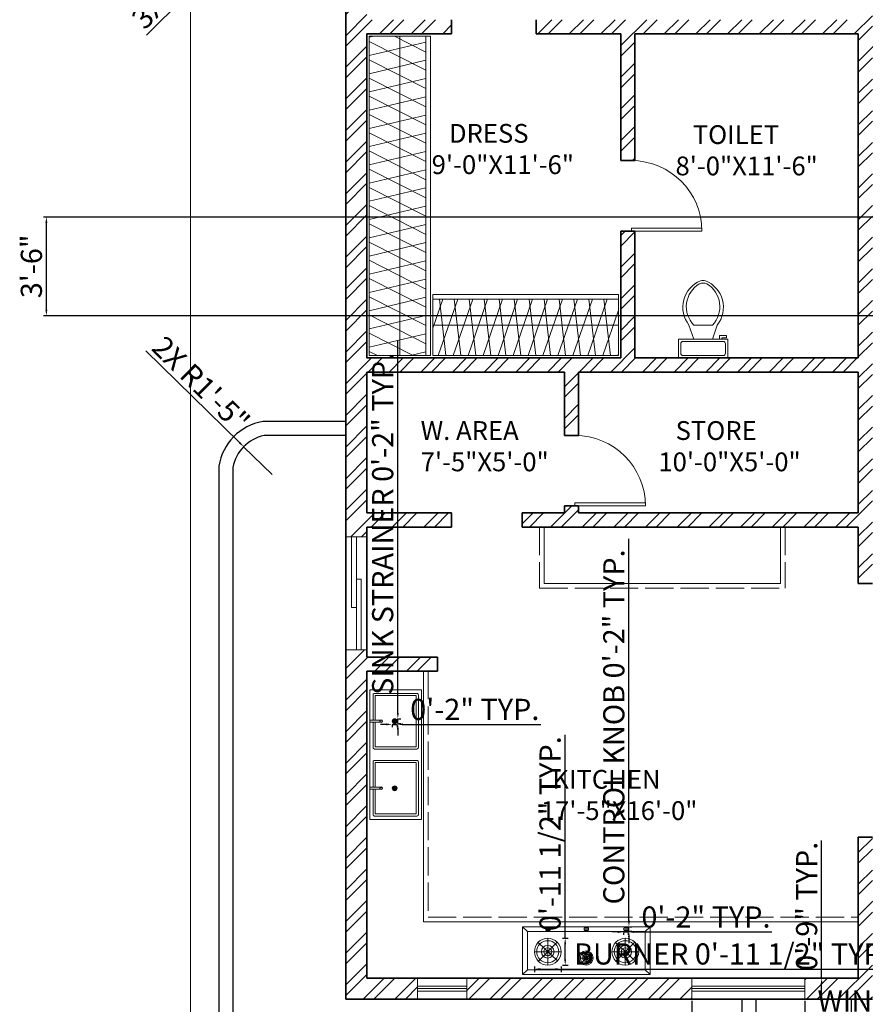
# Model space of a CAD drawing. Units: inches. Extents: x 155 to 1269, y 1260 to 2528.
# Tile 2 of 6: x 155 to 514, y 1484 to 1903. Entities that reach past the tile are written whole.
import ezdxf

# ---------------------------------------------------------------- set-up
doc = ezdxf.new("R2010")
doc.units = ezdxf.units.IN
doc.linetypes.add('ACAD_ISO02W100', pattern=[15, 12, -3])
for name, color, linetype, lineweight in [('A-ANNO-DIMS', 2, 'Continuous', 18), ('A-AREA-IDEN', 7, 'Continuous', 18), ('A-DOOR', 3, 'Continuous', 18), ('A-EQPM', 8, 'Continuous', 18), ('A-FLOR-CASE', 9, 'Continuous', 18), ('A-FLOR-CASE-HIDN', 9, 'ACAD_ISO02W100', 13), ('A-FLOR-CASE-PATT', 252, 'Continuous', 13), ('A-FLOR-EDGE', 7, 'Continuous', 25), ('A-FLOR-FIXT', 9, 'Continuous', 18), ('A-GLAZ', 244, 'Continuous', 18), ('A-WALL', 7, 'Continuous', 35), ('A-WALL-PATT', 252, 'Continuous', 13), ('C-PROP', 8, 'Continuous', 18)]:
    doc.layers.add(name, color=color, linetype=linetype, lineweight=lineweight)
doc.styles.get("Standard").update_dxf_attribs({"font": 'arial.ttf'})
doc.dimstyles.new('ISO-25', dxfattribs={"dimtxt": 9, "dimasz": 2.5, "dimexe": 1.25, "dimexo": 0.625, "dimtad": 1, "dimlunit": 3, "dimtxsty": 'Standard', "dimcen": 2.5, "dimadec": 0, "dimazin": 0, "dimtfac": 1, "dimtmove": 0, "dimatfit": 3, "dimfxl": 1, "dimarcsym": 0})

# ---------------------------------------------------------------- blocks, each defined once
blk = doc.blocks.new('*U2')
for p, q in [((0, 0), (0, -6)), ((-40, 0), (-40, -6))]:
    blk.add_line(p, q)
blk.add_lwpolyline([(0, 0), (0, 40), (-1.75, 40), (-1.75, 0)], close=True)
blk.add_arc((0, 0), 40, 90, 180)
blk = doc.blocks.new('*U8')
for p, q in [((9.5, -6), (9.5, -2)), ((-8, -8.5), (-8, -8)), ((-7, -8), (-7, -9.5)), ((-4, -8), (-6, -14)), ((4, -8), (6, -14)), ((-10, -8.5), (-8, -8.5)), ((-10, -9.5), (-10, -8.5)), ((-7, -9.5), (-10, -9.5)), ((4, -14), (-4, -14))]:
    blk.add_line(p, q)
blk.add_lwpolyline([(10.5, -8), (10.5, 0), (-10.5, 0), (-10.5, -8)], close=True)
for points in [[(-9.5, -2), (-9.5, -6)], [(8.5, -1), (-8.5, -1)], [(-8.5, -7), (8.5, -7)]]:
    blk.add_lwpolyline(points)
for centre, radius, start, end in [((-8.62, -1.88), 0.884, 81.8699, 188.1301), ((8.62, -1.88), 0.884, 351.8699, 98.1301), ((-8.62, -6.12), 0.884, 171.8699, 278.1301), ((8.62, -6.12), 0.884, 261.8699, 8.1301), ((3.52, -21.58), 12.17, 141.4691, 247.9714), ((4.2, -21.82), 11.33, 136.3677, 238.9468), ((-3.52, -21.58), 12.17, 292.0284, 38.5307), ((-4.2, -21.82), 11.33, 301.053, 43.6321), ((0, -27.88), 4, 245.7318, 294.2682), ((0, -29), 4, 254.8605, 285.1395)]:
    blk.add_arc(centre, radius, start, end)
blk = doc.blocks.new('WIN-21IN')
for p, q in [((21, 5.5), (0, 5.5)), ((21, 4.5), (0, 4.5)), ((21, 3.5), (0, 3.5))]:
    blk.add_line(p, q)
blk.add_lwpolyline([(0, 9), (21, 9), (21, 0), (0, 0)], close=True)
blk = doc.blocks.new('WIN-48IN')
for p, q in [((0, 5.5), (48, 5.5)), ((0, 4.5), (48, 4.5)), ((0, 3.5), (48, 3.5))]:
    blk.add_line(p, q)
blk.add_lwpolyline([(0, 9), (48, 9), (48, 0), (0, 0)], close=True)
blk = doc.blocks.new('COOKTOP-BURNER')
for p, q in [((9.85, 1.8), (1.54, 9.59)), ((1.69, 1.65), (9.7, 9.74)), ((5.69, 11.39), (5.69, 0)), ((0, 5.69), (11.39, 5.69))]:
    blk.add_line(p, q)
for radius in [5.69, 4.69, 2.69, 1.69]:
    blk.add_circle((5.69, 5.69), radius)
blk = doc.blocks.new('COOKTOP-KNOB')
for p, q in [((-0.93, 0.3), (0.93, 0.3)), ((-0.93, -0.3), (0.93, -0.3))]:
    blk.add_line(p, q)
blk.add_circle((0, 0), 0.979)
for radius, start, end in [(0.879, 19.9469, 160.0531), (0.579, 31.1844, 148.8156), (0.479, 38.7415, 141.2585), (0.879, 199.9469, 340.0531), (0.579, 211.1844, 328.8156), (0.479, 218.7415, 321.2585)]:
    blk.add_arc((0, 0), radius, start, end)
blk = doc.blocks.new('SINK-STRAINER')
for p, q in [((-1.03, 0), (1.03, 0)), ((0.77, -0.69), (-0.77, 0.69)), ((-0.65, -0.8), (0.65, 0.8)), ((0, 1.03), (0, -1.03))]:
    blk.add_line(p, q)
for radius in [1.03, 0.831, 0.731]:
    blk.add_circle((0, 0), radius)
blk = doc.blocks.new('*D30')
at = {"layer": 'A-ANNO-DIMS', "color": 0, "lineweight": -2, "transparency": 16777216}
for p, q in [((413.86, 1519.56), (413.86, 1682.15)), ((413.86, 1515.1), (413.86, 1517.06)), ((414.19, 1517.06), (415.11, 1517.06)), ((414.19, 1515.1), (415.11, 1515.1)), ((413.86, 1512.6), (413.86, 1510.1))]:
    blk.add_line(p, q, dxfattribs=at)
at = {"layer": 'A-ANNO-DIMS', "color": 0, "transparency": 16777216}
for points in [[(413.44, 1519.56), (414.28, 1519.56), (413.86, 1517.06)], [(413.44, 1512.6), (414.28, 1512.6), (413.86, 1515.1)]]:
    blk.add_solid(points, dxfattribs=at)
at = {"layer": 'Defpoints', "color": 0, "transparency": 16777216}
for p in [(413.57, 1517.06), (413.57, 1515.1), (413.86, 1517.06)]:
    blk.add_point(p, dxfattribs=at)
at = {"layer": 'A-ANNO-DIMS', "color": 0, "transparency": 16777216, "insert": (408.58, 1602.1), "char_height": 9, "attachment_point": 5, "rotation": 90}
blk.add_mtext('CONTROL KNOB 0\'-2" TYP.', dxfattribs=at)
blk = doc.blocks.new('*D31')
at = {"layer": 'A-ANNO-DIMS', "color": 0, "lineweight": -2, "transparency": 16777216}
for p, q in [((409.11, 1514.8), (406.61, 1514.8)), ((411.61, 1514.8), (413.57, 1514.8)), ((411.61, 1514.47), (411.61, 1513.55)), ((413.57, 1514.47), (413.57, 1513.55)), ((416.07, 1514.8), (474.68, 1514.8))]:
    blk.add_line(p, q, dxfattribs=at)
at = {"layer": 'A-ANNO-DIMS', "color": 0, "transparency": 16777216}
for points in [[(409.11, 1515.22), (409.11, 1514.39), (411.61, 1514.8)], [(416.07, 1515.22), (416.07, 1514.39), (413.57, 1514.8)]]:
    blk.add_solid(points, dxfattribs=at)
at = {"layer": 'Defpoints', "color": 0, "transparency": 16777216}
for p in [(411.61, 1515.1), (413.57, 1515.1), (413.57, 1514.8)]:
    blk.add_point(p, dxfattribs=at)
at = {"layer": 'A-ANNO-DIMS', "color": 0, "transparency": 16777216, "insert": (446.62, 1520.02), "char_height": 9, "attachment_point": 5}
blk.add_mtext('0\'-2" TYP.', dxfattribs=at)
blk = doc.blocks.new('*D34')
at = {"layer": 'A-ANNO-DIMS', "color": 0, "lineweight": -2, "transparency": 16777216}
for p, q in [((440.63, 1485.56), (440.63, 1477.73)), ((488.63, 1485.56), (488.63, 1477.73)), ((443.13, 1478.98), (486.13, 1478.98)), ((488.63, 1478.98), (606.27, 1478.98))]:
    blk.add_line(p, q, dxfattribs=at)
at = {"layer": 'A-ANNO-DIMS', "color": 0, "transparency": 16777216}
for points in [[(443.13, 1479.4), (443.13, 1478.56), (440.63, 1478.98)], [(486.13, 1479.4), (486.13, 1478.56), (488.63, 1478.98)]]:
    blk.add_solid(points, dxfattribs=at)
at = {"layer": 'Defpoints', "color": 0, "transparency": 16777216}
for p in [(440.63, 1486.18), (488.63, 1486.18), (488.63, 1478.98)]:
    blk.add_point(p, dxfattribs=at)
at = {"layer": 'A-ANNO-DIMS', "color": 0, "transparency": 16777216, "insert": (548.7, 1484.26), "char_height": 9, "attachment_point": 5}
blk.add_mtext('WINDOW 4\'-0" TYP.', dxfattribs=at)
blk = doc.blocks.new('*D35')
at = {"layer": 'A-ANNO-DIMS', "color": 0, "lineweight": -2, "transparency": 16777216}
for p, q in [((495.83, 1495.18), (495.83, 1553.79)), ((489.26, 1495.18), (497.08, 1495.18)), ((495.83, 1488.68), (495.83, 1492.68)), ((489.26, 1486.18), (497.08, 1486.18))]:
    blk.add_line(p, q, dxfattribs=at)
at = {"layer": 'A-ANNO-DIMS', "color": 0, "transparency": 16777216}
for points in [[(495.41, 1492.68), (496.25, 1492.68), (495.83, 1495.18)], [(495.41, 1488.68), (496.25, 1488.68), (495.83, 1486.18)]]:
    blk.add_solid(points, dxfattribs=at)
at = {"layer": 'Defpoints', "color": 0, "transparency": 16777216}
for p in [(488.63, 1495.18), (495.83, 1495.18), (488.63, 1486.18)]:
    blk.add_point(p, dxfattribs=at)
at = {"layer": 'A-ANNO-DIMS', "color": 0, "transparency": 16777216, "insert": (490.61, 1525.74), "char_height": 9, "attachment_point": 5, "rotation": 90}
blk.add_mtext('0\'-9" TYP.', dxfattribs=at)
blk = doc.blocks.new('*D36')
at = {"layer": 'A-ANNO-DIMS', "color": 0, "lineweight": -2, "transparency": 16777216}
for p, q in [((373.64, 1500.1), (373.64, 1497.76)), ((376.14, 1499.01), (382.53, 1499.01)), ((385.03, 1500.1), (385.03, 1497.76)), ((385.03, 1499.01), (527.79, 1499.01))]:
    blk.add_line(p, q, dxfattribs=at)
at = {"layer": 'A-ANNO-DIMS', "color": 0, "transparency": 16777216}
for points in [[(376.14, 1499.43), (376.14, 1498.6), (373.64, 1499.01)], [(382.53, 1499.43), (382.53, 1498.6), (385.03, 1499.01)]]:
    blk.add_solid(points, dxfattribs=at)
at = {"layer": 'Defpoints', "color": 0, "transparency": 16777216}
for p in [(373.64, 1500.72), (385.03, 1500.72), (385.03, 1499.01)]:
    blk.add_point(p, dxfattribs=at)
at = {"layer": 'A-ANNO-DIMS', "color": 0, "transparency": 16777216, "insert": (457.66, 1504.29), "char_height": 9, "attachment_point": 5}
blk.add_mtext('BURNER 0\'-11 1/2" TYP.', dxfattribs=at)
blk = doc.blocks.new('*D37')
at = {"layer": 'A-ANNO-DIMS', "color": 0, "lineweight": -2, "transparency": 16777216}
for p, q in [((386.74, 1512.11), (386.74, 1598.68)), ((385.65, 1512.11), (387.99, 1512.11)), ((386.74, 1503.22), (386.74, 1509.61)), ((385.65, 1500.72), (387.99, 1500.72))]:
    blk.add_line(p, q, dxfattribs=at)
at = {"layer": 'A-ANNO-DIMS', "color": 0, "transparency": 16777216}
for points in [[(386.32, 1509.61), (387.15, 1509.61), (386.74, 1512.11)], [(386.32, 1503.22), (387.15, 1503.22), (386.74, 1500.72)]]:
    blk.add_solid(points, dxfattribs=at)
at = {"layer": 'Defpoints', "color": 0, "transparency": 16777216}
for p in [(385.03, 1512.11), (386.74, 1512.11), (385.03, 1500.72)]:
    blk.add_point(p, dxfattribs=at)
at = {"layer": 'A-ANNO-DIMS', "color": 0, "transparency": 16777216, "insert": (381.46, 1556.65), "char_height": 9, "attachment_point": 5, "rotation": 90}
blk.add_mtext('0\'-11 1/2" TYP.', dxfattribs=at)
blk = doc.blocks.new('*D38')
at = {"layer": 'A-ANNO-DIMS', "color": 0, "lineweight": -2, "transparency": 16777216}
for p, q in [((315.54, 1608.06), (315.54, 1766.53)), ((315.54, 1603.5), (315.54, 1605.56)), ((315.86, 1605.56), (316.79, 1605.56)), ((315.86, 1603.5), (316.79, 1603.5)), ((315.54, 1601), (315.54, 1598.5))]:
    blk.add_line(p, q, dxfattribs=at)
at = {"layer": 'A-ANNO-DIMS', "color": 0, "transparency": 16777216}
for points in [[(315.13, 1608.06), (315.96, 1608.06), (315.54, 1605.56)], [(315.13, 1601), (315.96, 1601), (315.54, 1603.5)]]:
    blk.add_solid(points, dxfattribs=at)
at = {"layer": 'Defpoints', "color": 0, "transparency": 16777216}
for p in [(315.23, 1605.56), (315.54, 1605.56), (315.23, 1603.5)]:
    blk.add_point(p, dxfattribs=at)
at = {"layer": 'A-ANNO-DIMS', "color": 0, "transparency": 16777216, "insert": (310.26, 1688.55), "char_height": 9, "attachment_point": 5, "rotation": 90}
blk.add_mtext('SINK STRAINER 0\'-2" TYP.', dxfattribs=at)
blk = doc.blocks.new('*D39')
at = {"layer": 'A-ANNO-DIMS', "color": 0, "lineweight": -2, "transparency": 16777216}
for p, q in [((310.67, 1603.19), (308.17, 1603.19)), ((313.17, 1603.19), (315.23, 1603.19)), ((313.17, 1602.87), (313.17, 1601.94)), ((315.23, 1602.87), (315.23, 1601.94)), ((317.73, 1603.19), (376.34, 1603.19))]:
    blk.add_line(p, q, dxfattribs=at)
at = {"layer": 'A-ANNO-DIMS', "color": 0, "transparency": 16777216}
for points in [[(310.67, 1603.61), (310.67, 1602.77), (313.17, 1603.19)], [(317.73, 1603.61), (317.73, 1602.77), (315.23, 1603.19)]]:
    blk.add_solid(points, dxfattribs=at)
at = {"layer": 'Defpoints', "color": 0, "transparency": 16777216}
for p in [(313.17, 1603.5), (315.23, 1603.5), (315.23, 1603.19)]:
    blk.add_point(p, dxfattribs=at)
at = {"layer": 'A-ANNO-DIMS', "color": 0, "transparency": 16777216, "insert": (348.29, 1608.41), "char_height": 9, "attachment_point": 5}
blk.add_mtext('0\'-2" TYP.', dxfattribs=at)
blk = doc.blocks.new('*D46')
at = {"layer": 'A-ANNO-DIMS', "color": 0, "lineweight": -2, "transparency": 16777216}
for p, q in [((1009.77, 1819.18), (164.8, 1819.18)), ((166.05, 1779.68), (166.05, 1816.68)), ((1015.06, 1777.18), (164.8, 1777.18))]:
    blk.add_line(p, q, dxfattribs=at)
at = {"layer": 'A-ANNO-DIMS', "color": 0, "transparency": 16777216}
for points in [[(165.63, 1816.68), (166.46, 1816.68), (166.05, 1819.18)], [(165.63, 1779.68), (166.46, 1779.68), (166.05, 1777.18)]]:
    blk.add_solid(points, dxfattribs=at)
at = {"layer": 'Defpoints', "color": 0, "transparency": 16777216}
for p in [(166.05, 1819.18), (1010.4, 1819.18), (1015.68, 1777.18)]:
    blk.add_point(p, dxfattribs=at)
at = {"layer": 'A-ANNO-DIMS', "color": 0, "transparency": 16777216, "insert": (160.82, 1798.18), "char_height": 9, "attachment_point": 5, "rotation": 90}
blk.add_mtext('3\'-6"', dxfattribs=at)
blk = doc.blocks.new('*D55')
at = {"layer": 'A-ANNO-DIMS', "color": 0, "lineweight": -2, "transparency": 16777216}
for p, q in [((208.3, 1762.14), (248.17, 1723.13)), ((262.1, 1709.5), (249.96, 1721.38))]:
    blk.add_line(p, q, dxfattribs=at)
at = {"layer": 'A-ANNO-DIMS', "color": 0, "transparency": 16777216}
blk.add_solid([(248.46, 1723.43), (247.88, 1722.84), (249.96, 1721.38)], dxfattribs=at)
at = {"layer": 'Defpoints', "color": 0, "transparency": 16777216}
for p in [(249.96, 1721.38), (262.1, 1709.5)]:
    blk.add_point(p, dxfattribs=at)
at = {"layer": 'A-ANNO-DIMS', "color": 0, "transparency": 16777216, "insert": (230.99, 1747.24), "char_height": 9, "attachment_point": 5, "rotation": 315.6281}
blk.add_mtext('2X R1\'-5"', dxfattribs=at)
blk = doc.blocks.new('*D56')
at = {"layer": 'A-ANNO-DIMS', "color": 0, "lineweight": -2, "transparency": 16777216}
for p, q in [((260.38, 1948.16), (249.76, 1937.58)), ((208.58, 1896.56), (247.98, 1935.81))]:
    blk.add_line(p, q, dxfattribs=at)
at = {"layer": 'A-ANNO-DIMS', "color": 0, "transparency": 16777216}
blk.add_solid([(247.69, 1936.11), (248.28, 1935.52), (249.76, 1937.58)], dxfattribs=at)
at = {"layer": 'Defpoints', "color": 0, "transparency": 16777216}
for p in [(260.38, 1948.16), (249.76, 1937.58)]:
    blk.add_point(p, dxfattribs=at)
at = {"layer": 'A-ANNO-DIMS', "color": 0, "transparency": 16777216, "insert": (223.71, 1919), "char_height": 9, "attachment_point": 5, "rotation": 44.8922}
blk.add_mtext('3X R1\'-3"', dxfattribs=at)

msp = doc.modelspace()

# ---------------------------------------------------------------- hatches: boundary and pattern name
at = {"layer": 'A-FLOR-CASE-PATT'}
h = msp.add_hatch(dxfattribs=at)
h.set_pattern_fill('ANSI31', color=256, scale=2.1772, angle=107.975, style=0)
h.paths.add_polyline_path([(303.397, 1760.181), (327.397, 1760.181), (327.397, 1896.181), (303.397, 1896.181)])
h = msp.add_hatch(dxfattribs=at)
h.set_pattern_fill('ANSI31', color=256, scale=2.37783, angle=-31.6302, style=0)
h.paths.add_polyline_path([(303.397, 1760.181), (327.397, 1760.181), (327.397, 1896.181), (303.397, 1896.181)])
h = msp.add_hatch(dxfattribs=at)
h.set_pattern_fill('ANSI31', color=256, scale=1.89486, angle=25.9917, style=0)
h.paths.add_polyline_path([(330.397, 1760.181), (409.397, 1760.181), (409.397, 1784.181), (330.397, 1784.181)])
h = msp.add_hatch(dxfattribs=at)
h.set_pattern_fill('ANSI31', color=256, scale=1.99071, angle=51.6389, style=0)
h.paths.add_polyline_path([(330.397, 1760.181), (409.397, 1760.181), (409.397, 1784.181), (330.397, 1784.181)])
at = {"layer": 'A-WALL-PATT'}
h = msp.add_hatch(dxfattribs=at)
h.set_pattern_fill('ANSI32', color=256)
h.paths.add_polyline_path([(614.897, 1534.181), (593.397, 1534.181), (593.397, 1555.181), (589.397, 1555.181), (589.397, 1534.181), (517.397, 1534.181), (517.397, 1555.181), (511.397, 1555.181), (511.397, 1495.181), (488.631, 1495.181), (488.631, 1486.181), (517.397, 1486.181), (517.397, 1525.181), (614.897, 1525.181)])
h.paths.add_polyline_path([(440.631, 1495.181), (344.954, 1495.181), (344.954, 1486.181), (440.631, 1486.181)])
h.paths.add_polyline_path([(323.954, 1495.181), (302.397, 1495.181), (302.397, 1625.863), (332.397, 1625.863), (332.397, 1631.863), (302.397, 1631.863), (302.397, 1634.984), (293.397, 1634.984), (293.397, 1486.181), (323.954, 1486.181)])
h.paths.add_polyline_path([(302.397, 1753.181), (386.397, 1753.181), (386.397, 1726.181), (392.397, 1726.181), (392.397, 1753.181), (511.397, 1753.181), (511.397, 1693.181), (392.397, 1693.181), (392.397, 1696.181), (386.397, 1696.181), (386.397, 1693.181), (368.397, 1693.181), (368.397, 1687.181), (511.397, 1687.181), (511.397, 1663.181), (517.397, 1663.181), (517.397, 1891.181), (539.397, 1891.181), (539.397, 1897.181), (517.397, 1897.181), (517.397, 2050.181), (511.397, 2050.181), (511.397, 1903.181), (374.397, 1903.181), (374.397, 1897.181), (410.397, 1897.181), (410.397, 1843.181), (416.397, 1843.181), (416.397, 1897.181), (511.397, 1897.181), (511.397, 1759.181), (416.397, 1759.181), (416.397, 1813.181), (410.397, 1813.181), (410.397, 1759.181), (302.397, 1759.181), (302.397, 1897.181), (338.397, 1897.181), (338.397, 1903.181), (302.397, 1903.181), (302.397, 1935.29), (293.397, 1935.29), (293.397, 1682.984), (302.397, 1682.984), (302.397, 1687.181), (338.397, 1687.181), (338.397, 1693.181), (302.397, 1693.181)])
h.paths.add_polyline_path([(645.397, 1897.181), (623.397, 1897.181), (623.397, 1891.181), (645.397, 1891.181)])
h.paths.add_polyline_path([(678.397, 1897.181), (669.397, 1897.181), (669.397, 1891.181), (678.397, 1891.181)])
h.paths.add_polyline_path([(696.397, 1897.181), (687.397, 1897.181), (687.397, 1891.181), (696.397, 1891.181)])
h.paths.add_polyline_path([(714.397, 1897.181), (705.397, 1897.181), (705.397, 1891.181), (714.397, 1891.181)])
h.paths.add_polyline_path([(732.397, 1897.181), (723.397, 1897.181), (723.397, 1891.181), (732.397, 1891.181)])
h.paths.add_polyline_path([(302.397, 2033.891), (293.397, 2033.891), (293.397, 1959.29), (302.397, 1959.29)], flags=17)
h.paths.add_polyline_path([(302.397, 2089.181), (511.397, 2089.181), (511.397, 2086.181), (517.397, 2086.181), (517.397, 2089.181), (527.397, 2089.181), (527.397, 2095.181), (302.397, 2095.181), (302.397, 2145.471), (293.397, 2145.471), (293.397, 2057.891), (302.397, 2057.891)])
h.paths.add_polyline_path([(773.397, 2095.181), (572.397, 2095.181), (572.397, 2308.181), (613.397, 2308.181), (613.397, 2443.181), (557.897, 2443.181), (557.897, 2434.181), (604.397, 2434.181), (604.397, 2314.181), (490.397, 2314.181), (490.397, 2359.181), (484.397, 2359.181), (484.397, 2314.181), (374.397, 2314.181), (374.397, 2308.181), (566.397, 2308.181), (566.397, 2095.181), (563.397, 2095.181), (563.397, 2089.181), (773.397, 2089.181)])
h.paths.add_polyline_path([(1070.397, 2147.681), (1061.397, 2147.681), (1061.397, 2095.181), (857.397, 2095.181), (857.397, 2089.181), (868.397, 2089.181), (868.397, 2086.181), (874.397, 2086.181), (874.397, 2089.181), (1061.397, 2089.181), (1061.397, 2050.181), (1070.397, 2050.181)])
h.paths.add_polyline_path([(821.397, 2095.181), (818.397, 2095.181), (818.397, 2308.181), (1022.397, 2308.181), (1022.397, 2314.181), (940.397, 2314.181), (940.397, 2434.181), (1077.397, 2434.181), (1077.397, 2389.181), (1083.397, 2389.181), (1083.397, 2434.181), (1129.897, 2434.181), (1129.897, 2443.181), (887.897, 2443.181), (887.897, 2434.181), (934.397, 2434.181), (934.397, 2314.181), (820.397, 2314.181), (820.397, 2359.181), (814.397, 2359.181), (814.397, 2314.181), (809.397, 2314.181), (809.397, 2308.181), (812.397, 2308.181), (812.397, 2095.181), (809.397, 2095.181), (809.397, 2089.181), (821.397, 2089.181)])
h.paths.add_polyline_path([(874.397, 2050.181), (868.397, 2050.181), (868.397, 1741.181), (877.397, 1741.181), (877.397, 1747.181), (892.397, 1747.181), (892.397, 1753.181), (874.397, 1753.181), (874.397, 1819.181), (940.397, 1819.181), (940.397, 1753.181), (922.397, 1753.181), (922.397, 1747.181), (946.397, 1747.181), (946.397, 1819.181), (1151.397, 1819.181), (1151.397, 1683.181), (931.397, 1683.181), (931.397, 1677.181), (1064.397, 1677.181), (1064.397, 1495.181), (877.397, 1495.181), (877.397, 1638.181), (868.397, 1638.181), (868.397, 1534.181), (796.397, 1534.181), (796.397, 1555.181), (792.397, 1555.181), (792.397, 1534.181), (770.897, 1534.181), (770.897, 1525.181), (868.397, 1525.181), (868.397, 1486.181), (1073.397, 1486.181), (1073.397, 1677.181), (1160.397, 1677.181), (1160.397, 1825.181), (1070.397, 1825.181), (1070.397, 1942.181), (1061.397, 1942.181), (1061.397, 1903.181), (913.397, 1903.181), (913.397, 1897.181), (1061.397, 1897.181), (1061.397, 1825.181), (957.406, 1825.181), (957.406, 1861.181), (951.406, 1861.181), (951.406, 1825.181), (874.397, 1825.181), (874.397, 1897.181), (877.397, 1897.181), (877.397, 1903.181), (874.397, 1903.181)])
h.paths.add_polyline_path([(1070.397, 2305.181), (1206.397, 2305.181), (1206.397, 2443.181), (1150.897, 2443.181), (1150.897, 2434.181), (1197.397, 2434.181), (1197.397, 2314.181), (1083.397, 2314.181), (1083.397, 2359.181), (1077.397, 2359.181), (1077.397, 2314.181), (1058.397, 2314.181), (1058.397, 2308.181), (1061.397, 2308.181), (1061.397, 2255.681), (1070.397, 2255.681)])
h.paths.add_polyline_path([(866.897, 2443.181), (673.397, 2443.181), (673.397, 2308.181), (773.397, 2308.181), (773.397, 2314.181), (682.397, 2314.181), (682.397, 2434.181), (814.397, 2434.181), (814.397, 2389.181), (818.897, 2389.181), (820.397, 2389.181), (820.397, 2434.181), (866.897, 2434.181)])
h.paths.add_polyline_path([(536.897, 2443.181), (293.397, 2443.181), (293.397, 2253.471), (302.397, 2253.471), (302.397, 2308.181), (338.397, 2308.181), (338.397, 2314.181), (302.397, 2314.181), (302.397, 2434.181), (484.397, 2434.181), (484.397, 2389.181), (490.397, 2389.181), (490.397, 2434.181), (536.897, 2434.181)])

# ---------------------------------------------------------------- linework, layer by layer
at = {"layer": 'A-EQPM'}
for p, q in [((370.638, 1515.057), (368.638, 1517.057)), ((420.827, 1515.057), (422.827, 1517.057)), ((397.8, 1501.671), (393.423, 1505.775)), ((393.5, 1501.592), (397.724, 1505.853)), ((395.612, 1506.723), (395.612, 1500.723)), ((392.612, 1503.723), (398.612, 1503.723)), ((370.638, 1498.725), (368.638, 1496.725)), ((420.827, 1498.725), (422.827, 1496.725))]:
    msp.add_line(p, q, dxfattribs=at)
for points in [[(368.638, 1517.057), (422.827, 1517.057), (422.827, 1496.725), (368.638, 1496.725)], [(370.638, 1515.057), (420.827, 1515.057), (420.827, 1498.725), (370.638, 1498.725)]]:
    msp.add_lwpolyline(points, close=True, dxfattribs=at)
for radius in [3, 2.473, 1.419, 0.892]:
    msp.add_circle((395.612, 1503.723), radius, dxfattribs=at)
at = {"layer": 'A-FLOR-CASE'}
for p, q in [((303.397, 1896.181), (303.397, 1760.181)), ((303.397, 1896.181), (329.397, 1896.181)), ((316.397, 1760.181), (316.397, 1896.181)), ((327.397, 1896.181), (327.397, 1760.181)), ((329.397, 1896.181), (329.397, 1760.181)), ((330.397, 1786.181), (330.397, 1760.181)), ((330.397, 1786.181), (409.397, 1786.181)), ((409.397, 1786.181), (409.397, 1760.181)), ((330.397, 1784.181), (409.397, 1784.181)), ((330.397, 1773.181), (409.397, 1773.181)), ((303.397, 1760.181), (329.397, 1760.181)), ((330.397, 1760.181), (409.397, 1760.181)), ((377.825, 1687.181), (377.825, 1663.181)), ((478.261, 1687.181), (478.261, 1663.181)), ((377.825, 1663.181), (478.261, 1663.181)), ((326.397, 1625.863), (326.397, 1519.181)), ((326.397, 1519.181), (511.397, 1519.181))]:
    msp.add_line(p, q, dxfattribs=at)
at = {"layer": 'A-FLOR-CASE-HIDN'}
for p, q in [((375.825, 1687.181), (375.825, 1661.181)), ((480.261, 1687.181), (480.261, 1661.181)), ((375.825, 1661.181), (480.261, 1661.181)), ((328.397, 1625.863), (328.397, 1521.181)), ((328.397, 1521.181), (511.397, 1521.181))]:
    msp.add_line(p, q, dxfattribs=at)
at = {"layer": 'A-FLOR-EDGE'}
for p, q in [((293.397, 1732.136), (258.058, 1732.136)), ((293.397, 1726.136), (258.631, 1726.136)), ((239.397, 1713.12), (239.397, 1404.446)), ((245.397, 1712.609), (245.397, 1404.556)), ((461.899, 1486.181), (461.899, 1404.585)), ((467.899, 1486.181), (467.899, 1404.435)), ((508.397, 1486.181), (508.397, 1384.181))]:
    msp.add_line(p, q, dxfattribs=at)
for radius, start, end in [(22.994, 100.13561, 170.94319), (16.994, 101.79532, 169.46111)]:
    msp.add_arc((262.105, 1709.501), radius, start, end, dxfattribs=at)
at = {"layer": 'A-FLOR-FIXT'}
for p, q in [((303.654, 1604.93), (308.022, 1604.93)), ((303.654, 1604.13), (308.022, 1604.13)), ((303.654, 1576.387), (308.022, 1576.387)), ((303.654, 1575.587), (308.022, 1575.587))]:
    msp.add_line(p, q, dxfattribs=at)
msp.add_lwpolyline([(303.654, 1617.88), (325.541, 1617.88), (325.541, 1562.637), (303.654, 1562.637)], close=True, dxfattribs=at)
for points in [[(305.039, 1604.93), (305.039, 1615.774, -0.4142136), (305.639, 1616.374), (323.664, 1616.374, -0.4142136), (324.264, 1615.774), (324.264, 1593.286, -0.4142136), (323.664, 1592.686), (305.639, 1592.686, -0.4142136), (305.039, 1593.286), (305.039, 1604.13)], [(305.039, 1575.587), (305.039, 1564.743, 0.4142136), (305.639, 1564.143), (323.664, 1564.143, 0.4142136), (324.264, 1564.743), (324.264, 1587.231, 0.4142136), (323.664, 1587.831), (305.639, 1587.831, 0.4142136), (305.039, 1587.231), (305.039, 1576.387)]]:
    msp.add_lwpolyline(points, format="xyb", dxfattribs=at)
for points in [[(305.939, 1604.93), (305.939, 1615.474), (323.364, 1615.474), (323.364, 1593.586), (305.939, 1593.586), (305.939, 1604.13)], [(305.939, 1575.587), (305.939, 1565.043), (323.364, 1565.043), (323.364, 1586.931), (305.939, 1586.931), (305.939, 1576.387)]]:
    msp.add_lwpolyline(points, dxfattribs=at)
for centre, radius in [((308.452, 1604.53), 0.587), ((308.452, 1604.53), 0.387), ((308.452, 1575.987), 0.587), ((308.452, 1575.987), 0.387)]:
    msp.add_circle(centre, radius, dxfattribs=at)
at = {"layer": 'A-GLAZ'}
for p, q in [((295.897, 1682.984), (295.897, 1652.984)), ((297.897, 1682.984), (297.897, 1634.984)), ((297.897, 1664.984), (299.897, 1664.984)), ((299.897, 1664.984), (299.897, 1634.984)), ((297.897, 1652.984), (295.897, 1652.984))]:
    msp.add_line(p, q, dxfattribs=at)
msp.add_lwpolyline([(293.397, 1682.984), (302.397, 1682.984), (302.397, 1634.984), (293.397, 1634.984)], close=True, dxfattribs=at)
at = {"layer": 'A-WALL'}
for p, q in [((293.397, 2443.181), (293.397, 1486.181)), ((338.397, 1897.181), (338.397, 1903.181)), ((374.397, 1897.181), (374.397, 1903.181)), ((302.397, 1897.181), (338.397, 1897.181)), ((302.397, 1897.181), (302.397, 1759.181)), ((374.397, 1897.181), (410.397, 1897.181)), ((410.397, 1897.181), (410.397, 1843.181)), ((416.397, 1897.181), (416.397, 1843.181)), ((416.397, 1897.181), (511.397, 1897.181)), ((511.397, 1897.181), (511.397, 1759.181)), ((410.397, 1843.181), (416.397, 1843.181)), ((410.397, 1813.181), (416.397, 1813.181)), ((410.397, 1813.181), (410.397, 1759.181)), ((416.397, 1813.181), (416.397, 1759.181)), ((302.397, 1759.181), (410.397, 1759.181)), ((416.397, 1759.181), (511.397, 1759.181)), ((302.397, 1753.181), (386.397, 1753.181)), ((302.397, 1753.181), (302.397, 1693.181)), ((386.397, 1753.181), (386.397, 1726.181)), ((392.397, 1753.181), (392.397, 1726.181)), ((392.397, 1753.181), (511.397, 1753.181)), ((511.397, 1753.181), (511.397, 1693.181)), ((386.397, 1726.181), (392.397, 1726.181)), ((386.397, 1696.181), (392.397, 1696.181)), ((386.397, 1696.181), (386.397, 1693.181)), ((392.397, 1696.181), (392.397, 1693.181)), ((302.397, 1693.181), (338.397, 1693.181)), ((338.397, 1693.181), (338.397, 1687.181)), ((368.397, 1693.181), (368.397, 1687.181)), ((368.397, 1693.181), (386.397, 1693.181)), ((392.397, 1693.181), (511.397, 1693.181)), ((302.397, 1687.181), (338.397, 1687.181)), ((302.397, 1687.181), (302.397, 1631.863)), ((368.397, 1687.181), (511.397, 1687.181)), ((511.397, 1687.181), (511.397, 1663.181)), ((511.397, 1663.181), (517.397, 1663.181)), ((302.397, 1631.863), (332.397, 1631.863)), ((332.397, 1631.863), (332.397, 1625.863)), ((302.397, 1625.863), (332.397, 1625.863)), ((302.397, 1625.863), (302.397, 1495.181)), ((511.397, 1555.181), (517.397, 1555.181)), ((511.397, 1555.181), (511.397, 1495.181)), ((302.397, 1495.181), (511.397, 1495.181)), ((293.397, 1486.181), (517.397, 1486.181))]:
    msp.add_line(p, q, dxfattribs=at)
at = {"layer": 'C-PROP'}
msp.add_line((227.397, 2455.181), (227.397, 1339.181), dxfattribs=at)

# ---------------------------------------------------------------- block references
at = {"layer": 'A-DOOR', "xscale": 0.7500000000000114, "yscale": 0.7500000000000114, "zscale": 0.7500000000000114, "rotation": 270}
for p in [(414.897, 1813.181), (390.897, 1696.181)]:
    msp.add_blockref('*U2', p, dxfattribs=at)
at = {"layer": 'A-EQPM'}
for name, p in [('COOKTOP-KNOB', (379.382, 1516.046)), ('COOKTOP-KNOB', (395.732, 1516.078)), ('COOKTOP-KNOB', (412.587, 1516.078)), ('COOKTOP-BURNER', (373.642, 1500.723)), ('COOKTOP-BURNER', (406.627, 1500.723))]:
    msp.add_blockref(name, p, dxfattribs=at)
at = {"layer": 'A-FLOR-FIXT', "rotation": 180}
msp.add_blockref('*U8', (445.396, 1759.181), dxfattribs=at)
at = {"layer": 'A-FLOR-FIXT'}
for p in [(314.202, 1604.53), (314.202, 1575.987)]:
    msp.add_blockref('SINK-STRAINER', p, dxfattribs=at)
at = {"layer": 'A-GLAZ'}
for name, p in [('WIN-21IN', (323.954, 1486.181)), ('WIN-48IN', (440.631, 1486.181))]:
    msp.add_blockref(name, p, dxfattribs=at)

# ---------------------------------------------------------------- texts
at = {"layer": 'A-AREA-IDEN', "char_height": 8, "attachment_point": 1}
for s, width, insert in [('   DRESS\\P9\'-0"X11\'-6"', 58.09546, (329.942, 1858.796)), ('   TOILET\\P8\'-0"X11\'-6"', 56.71156, (433.666, 1858.252)), ('W. AREA\\P7\'-5"X5\'-0"', 51.1877, (325.254, 1732.277)), ('   STORE\\P10\'-0"X5\'-0"', 57.88225, (426.375, 1732.277)), ('  KITCHEN\\P17\'-5"X16\'-0"', 62.56701, (376.379, 1583.805))]:
    msp.add_mtext_dynamic_manual_height_columns(s, width=width, gutter_width=12.5, heights=[0], dxfattribs=dict(at, insert=insert))

# ---------------------------------------------------------------- dimensions: what is measured, and where the dimension line sits
at = {"layer": 'A-ANNO-DIMS'}
for center, mpoint, text, picture, middle in [((260.376, 1948.157), (249.756, 1937.577), '3X <>', '*D56', (223.712, 1919.003)), ((262.105, 1709.501), (249.957, 1721.385), '2X <>', '*D55', (230.991, 1747.242))]:
    dim = msp.add_radius_dim(center=center, mpoint=mpoint, text=text, dimstyle='ISO-25', override={"dimdec": 1, "dimlfac": 1, "dimrnd": 0, "dimzin": 1, "dimdsep": 46, "dimlunit": 4, "dimfrac": 2}, dxfattribs=at)
    dim.commit()
    dim.dimension.update_dxf_attribs({"geometry": picture, "text_midpoint": middle})
dim = msp.add_linear_dim(base=(166.047, 1819.181), p1=(1015.681, 1777.181), p2=(1010.397, 1819.181), angle=90, dimstyle='ISO-25', override={"dimdec": 1, "dimlfac": 1, "dimrnd": 0, "dimzin": 1, "dimdsep": 46, "dimlunit": 4, "dimfrac": 2}, dxfattribs=at)
dim.commit()
dim.dimension.update_dxf_attribs({"geometry": '*D46', "text_midpoint": (160.824, 1798.181)})
for base, p1, p2, text, picture, middle in [((315.542, 1605.561), (315.233, 1603.499), (315.233, 1605.561), 'SINK STRAINER <> TYP.', '*D38', (310.264, 1688.546)), ((413.86, 1517.057), (413.566, 1515.099), (413.566, 1517.057), 'CONTROL KNOB <> TYP.', '*D30', (408.578, 1602.105)), ((386.738, 1512.111), (385.03, 1500.723), (385.03, 1512.111), '<> TYP.', '*D37', (381.459, 1556.647)), ((495.831, 1495.181), (488.631, 1486.181), (488.631, 1495.181), '<> TYP.', '*D35', (490.611, 1525.736))]:
    dim = msp.add_linear_dim(base=base, p1=p1, p2=p2, angle=90, text=text, dimstyle='ISO-25', override={"dimdec": 1, "dimlfac": 1, "dimrnd": 0, "dimzin": 1, "dimdsep": 46, "dimlunit": 4, "dimfrac": 2}, dxfattribs=at)
    dim.commit()
    dim.dimension.update_dxf_attribs({"geometry": picture, "text_midpoint": middle})
for base, p1, p2, text, picture, middle in [((315.233, 1603.189), (313.17, 1603.499), (315.233, 1603.499), '<> TYP.', '*D39', (348.288, 1608.409)), ((385.03, 1499.015), (373.642, 1500.723), (385.03, 1500.723), 'BURNER <> TYP.', '*D36', (457.659, 1504.293)), ((413.566, 1514.805), (411.607, 1515.099), (413.566, 1515.099), '<> TYP.', '*D31', (446.621, 1520.025)), ((488.631, 1478.981), (440.631, 1486.181), (488.631, 1486.181), 'WINDOW <> TYP.', '*D34', (548.7, 1484.262))]:
    dim = msp.add_linear_dim(base=base, p1=p1, p2=p2, text=text, dimstyle='ISO-25', override={"dimdec": 1, "dimlfac": 1, "dimrnd": 0, "dimzin": 1, "dimdsep": 46, "dimlunit": 4, "dimfrac": 2}, dxfattribs=at)
    dim.commit()
    dim.dimension.update_dxf_attribs({"geometry": picture, "text_midpoint": middle})

doc.saveas('drawing.dxf')
